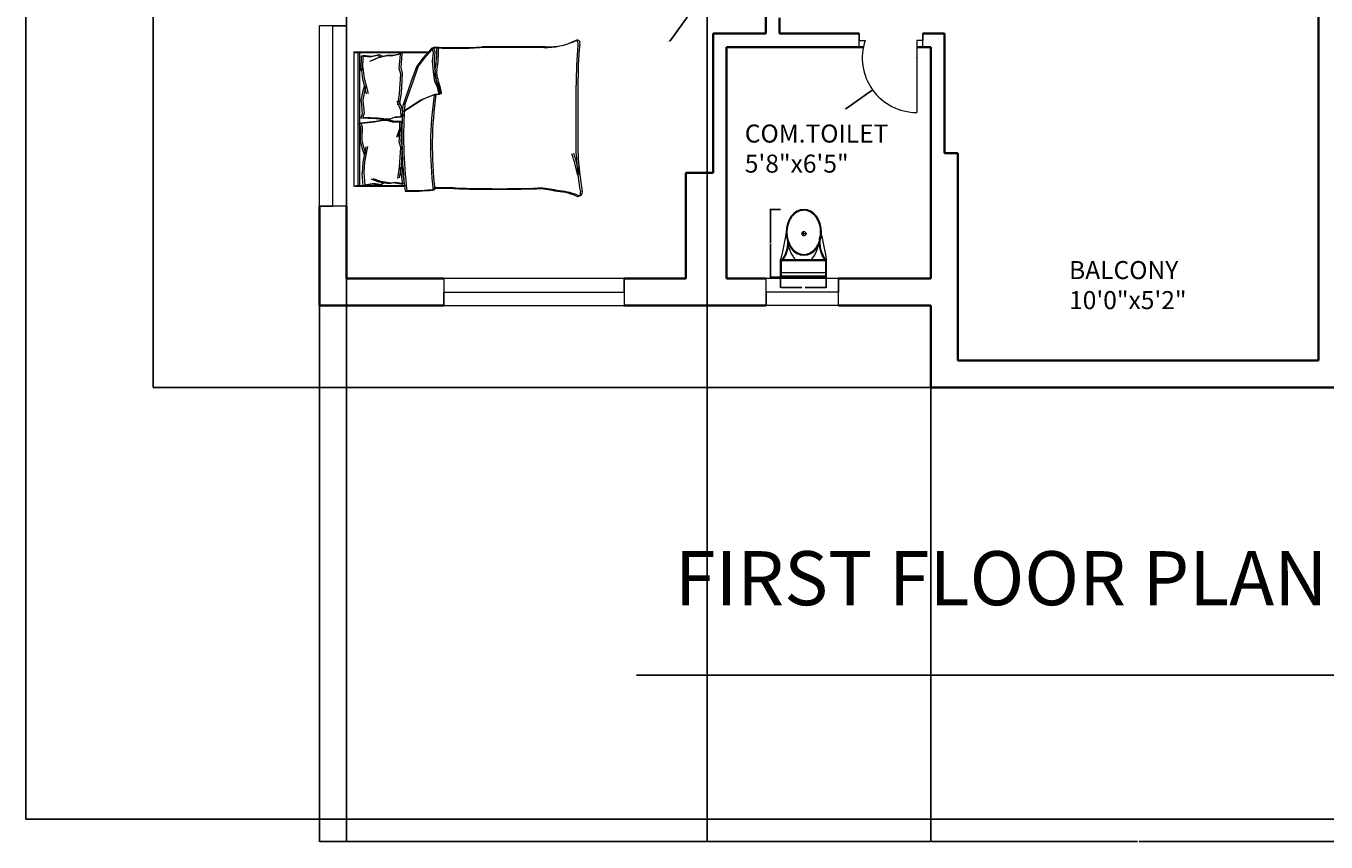
# Model space of a CAD drawing. Units: inches. Extents: x 1902 to 2626, y 1199 to 2408.
# Tile 1 of 9: x 1902 to 2334, y 1199 to 1470. Entities that reach past the tile are written whole.
import ezdxf

# ---------------------------------------------------------------- set-up
doc = ezdxf.new("R2010")
doc.units = ezdxf.units.IN
for name, color, linetype, lineweight in [('A-ANNO-DIMS', 2, 'Continuous', 18), ('A-ANNO-TTLB', 7, 'Continuous', 25), ('A-AREA-IDEN', 7, 'Continuous', 18), ('A-DOOR', 31, 'Continuous', 18), ('A-FLOR-FIXT', 9, 'Continuous', 18), ('A-FURN', 8, 'Continuous', 13), ('A-GLAZ', 181, 'Continuous', 18), ('A-WALL', 7, 'Continuous', 35)]:
    doc.layers.add(name, color=color, linetype=linetype, lineweight=lineweight)
doc.styles.get("Standard").update_dxf_attribs({"font": 'arial.ttf'})
doc.dimstyles.get("Standard").update_dxf_attribs({"dimtxt": 0.18, "dimasz": 0.18, "dimexe": 0.18, "dimexo": 0.0625, "dimgap": 0.09, "dimtad": 0, "dimtih": 1, "dimtoh": 1, "dimdec": 4, "dimzin": 0, "dimdsep": 46, "dimtxsty": 'Standard', "dimcen": 0.09, "dimadec": 0, "dimazin": 0, "dimtfac": 1, "dimtdec": 4, "dimtofl": 0, "dimtmove": 0, "dimatfit": 3, "dimfxl": 1, "dimtolj": 1, "dimtzin": 0, "dimarcsym": 0})

# ---------------------------------------------------------------- blocks, each defined once
blk = doc.blocks.new('A$C31115884')
for p, q in [((283, 498), (223, 498)), ((258, 466), (258, 523)), ((0, 200), (0, 0)), ((520, 200), (0, 200)), ((10, 190), (10, 10)), ((510, 190), (10, 190)), ((510, 10), (510, 190)), ((520, 0), (520, 200)), ((510, 54), (0, 54)), ((10, 10), (510, 10)), ((0, 0), (520, 0))]:
    blk.add_line(p, q)
blk.add_circle((256, 496), 23.6)
for centre, radius, start, end in [((2778, -205), 2807, 165.4549, 171.7133), ((-295, 403), 365, 324.2091, 9.3499), ((-295, 403), 375, 324.2091, 9.3499), ((806, 403), 365, 170.6501, 215.7909), ((3237, 905), 2807, 188.2867, 194.5451), ((384, 406), 293, 190.2774, 224.1564), ((139, 406), 293, 315.8436, 2.6563), ((806, 403), 375, 179.2036, 215.7909)]:
    blk.add_arc(centre, radius, start, end)
blk.add_ellipse((256, 510), major_axis=(0, -261), ratio=0.772727)
blk.add_open_spline([(256, 259), (263, 259), (270, 260), (288, 262), (299, 265), (320, 273), (330, 278), (350, 291), (360, 299), (378, 316), (386, 326), (402, 347), (409, 358), (421, 383), (427, 395), (436, 422), (440, 436), (445, 465), (447, 480), (448, 509), (448, 524), (445, 553), (443, 568), (436, 596), (432, 610), (422, 636), (416, 649), (402, 672), (395, 683), (379, 703), (370, 712), (351, 728), (341, 735), (321, 746), (310, 751), (289, 757), (278, 759), (256, 761), (245, 761), (223, 757), (212, 754), (191, 746), (181, 741), (161, 728), (151, 720), (133, 703), (125, 693), (110, 672), (103, 660), (90, 636), (85, 623), (76, 596), (72, 582), (67, 553), (66, 538), (64, 509), (65, 494), (68, 465), (70, 450), (77, 422), (81, 408), (91, 382), (97, 370), (111, 346), (118, 335), (135, 316), (144, 307), (162, 291), (172, 284), (193, 273), (203, 269), (225, 262), (236, 260), (250, 259), (253, 259), (256, 259)], degree=3, knots=[0, 0, 0, 0, 0.110105, 0.110105, 0.285049, 0.285049, 0.459994, 0.459994, 0.634938, 0.634938, 0.809882, 0.809882, 0.984827, 0.984827, 1.159771, 1.159771, 1.334715, 1.334715, 1.50966, 1.50966, 1.684604, 1.684604, 1.859549, 1.859549, 2.034493, 2.034493, 2.209437, 2.209437, 2.384382, 2.384382, 2.559326, 2.559326, 2.73427, 2.73427, 2.909215, 2.909215, 3.084159, 3.084159, 3.259103, 3.259103, 3.434048, 3.434048, 3.608992, 3.608992, 3.783936, 3.783936, 3.958881, 3.958881, 4.133825, 4.133825, 4.30877, 4.30877, 4.483714, 4.483714, 4.658658, 4.658658, 4.833603, 4.833603, 5.008547, 5.008547, 5.183491, 5.183491, 5.358436, 5.358436, 5.53338, 5.53338, 5.708324, 5.708324, 5.883269, 5.883269, 6.058213, 6.058213, 6.233158, 6.233158, 6.283185, 6.283185, 6.283185, 6.283185])
blk = doc.blocks.new('BED-DOUBLE')
for p, q in [((-0.01, 48.09), (0.59, 48.09)), ((-0.01, 48.09), (-0.01, 3.46)), ((-0.01, 47.87), (24.84, 47.87)), ((-0.01, 47.87), (24.84, 47.87)), ((0.59, 48.09), (25.44, 48.09)), ((0.59, 48.09), (25.44, 48.09)), ((1.43, 3.25), (1.43, 47.87)), ((1.43, 3.25), (1.43, 47.87)), ((2.02, 3.46), (2.02, 48.09)), ((2.02, 3.46), (2.02, 48.09)), ((25.9, 49.37), (22.87, 45.91)), ((25.9, 49.37), (22.87, 45.91)), ((26.5, 49.58), (23.46, 46.12)), ((26.5, 49.58), (23.46, 46.12)), ((27.53, 49.44), (25.9, 49.37, 3.61)), ((27.53, 49.44), (25.9, 49.37, 3.61)), ((26.48, 47.93), (25.9, 49.37)), ((26.48, 47.93), (25.9, 49.37)), ((26.19, 45.04), (26.48, 47.93)), ((26.19, 45.04), (26.48, 47.93)), ((28.13, 49.66), (26.5, 49.58, 3.61)), ((28.13, 49.66), (26.5, 49.58, 3.61)), ((27.08, 48.15), (26.5, 49.58)), ((27.08, 48.15), (26.5, 49.58)), ((26.79, 45.26), (27.08, 48.15)), ((26.79, 45.25), (27.08, 48.15)), ((2.38, 46.8), (2.29, 41.75)), ((2.38, 46.8), (2.29, 41.75)), ((2.38, 46.8), (5.38, 46.44)), ((2.38, 46.8), (5.38, 46.44)), ((2.98, 47.01), (2.89, 41.97)), ((2.98, 47.01), (2.89, 41.96)), ((2.98, 47.01), (5.98, 46.66)), ((2.98, 47.01), (5.98, 46.66)), ((7.7, 46.05), (5.2, 44.94)), ((7.7, 46.05), (5.2, 44.94)), ((5.38, 46.44), (7.78, 47)), ((5.38, 46.44), (7.78, 47)), ((8.3, 46.26), (5.8, 45.16)), ((8.3, 46.26), (5.8, 45.16)), ((5.98, 46.66), (8.38, 47.21)), ((5.98, 46.66), (8.38, 47.21)), ((11.04, 46.8), (7.7, 46.05)), ((11.04, 46.8), (7.7, 46.05)), ((7.78, 47), (8.76, 46.52)), ((7.78, 47), (8.76, 46.52)), ((11.64, 47.01), (8.3, 46.26)), ((11.64, 47.01), (8.3, 46.26)), ((8.38, 47.21), (9.35, 46.73)), ((8.38, 47.21), (9.35, 46.73)), ((12.54, 46.62), (11.04, 46.8)), ((12.54, 46.62), (11.04, 46.8)), ((13.14, 46.83), (11.64, 47.01)), ((13.14, 46.83), (11.64, 47.01)), ((15.47, 47.34), (12.54, 46.62)), ((15.47, 47.34), (12.54, 46.62)), ((16.07, 47.56), (13.14, 46.83)), ((16.07, 47.56), (13.14, 46.83)), ((15.09, 42.55), (15.47, 47.34)), ((15.09, 42.55), (15.47, 47.34)), ((15.69, 42.77), (16.07, 47.56)), ((15.69, 42.77), (16.07, 47.56)), ((21.44, 43.38), (19.56, 38.17)), ((21.44, 43.38), (19.56, 38.17)), ((22.87, 45.91), (20.84, 43.16)), ((22.87, 45.91), (20.84, 43.16)), ((23.46, 46.12), (21.44, 43.38)), ((23.46, 46.12), (21.44, 43.38)), ((26.48, 41.43), (26.19, 45.04)), ((26.48, 41.43), (26.19, 45.04)), ((27.08, 41.64), (26.79, 45.26)), ((27.08, 41.64), (26.79, 45.25)), ((2.29, 41.75), (2.37, 42.69)), ((2.29, 41.75), (2.37, 42.69)), ((2.37, 42.69), (2.86, 39.14)), ((2.37, 42.69), (2.86, 39.14)), ((2.86, 39.14), (4.12, 34.08)), ((2.86, 39.14), (4.12, 34.08)), ((2.89, 41.97), (2.97, 42.9)), ((2.89, 41.96), (2.97, 42.9)), ((2.97, 42.9), (3.46, 39.36)), ((2.97, 42.9), (3.46, 39.35)), ((3.46, 39.36), (4.72, 34.29)), ((3.46, 39.35), (4.72, 34.29)), ((15.61, 40.72), (15.09, 42.55)), ((15.61, 40.72), (15.09, 42.55)), ((15.21, 34.18), (15.61, 40.72)), ((15.21, 34.18), (15.61, 40.72)), ((16.21, 40.93), (15.69, 42.77)), ((16.21, 40.93), (15.69, 42.77)), ((15.81, 34.39), (16.21, 40.93)), ((15.81, 34.39), (16.21, 40.93)), ((20.84, 43.16), (18.97, 37.96)), ((20.84, 43.16), (18.97, 37.96)), ((26.91, 38.25), (26.48, 41.43)), ((26.91, 38.24), (26.48, 41.43)), ((27.51, 38.46), (27.08, 41.64)), ((27.51, 38.46), (27.08, 41.64)), ((2.87, 34.68), (2.36, 31.94)), ((2.87, 34.68), (2.36, 31.94)), ((3.42, 36.61), (2.87, 34.68)), ((3.42, 36.61), (2.87, 34.68)), ((3.47, 34.89), (2.96, 32.16)), ((3.47, 34.89), (2.96, 32.16)), ((4.02, 36.82), (3.47, 34.89)), ((4.02, 36.82), (3.47, 34.89)), ((18.97, 37.96), (16.23, 30.17)), ((18.97, 37.96), (16.23, 30.17)), ((19.56, 38.17), (16.82, 30.38)), ((19.56, 38.17), (16.82, 30.38)), ((27.78, 36.37), (26.91, 38.25)), ((27.78, 36.36), (26.91, 38.24)), ((28.38, 36.58), (27.51, 38.46)), ((28.38, 36.58), (27.51, 38.46)), ((28.36, 34.05), (27.78, 36.37)), ((28.36, 34.05), (27.78, 36.36)), ((28.96, 34.26), (28.38, 36.58)), ((28.96, 34.26), (28.38, 36.58)), ((73.99, 14.07), (73.99, 37.05)), ((73.99, 14.07), (73.99, 37.05)), ((74.59, 14.28), (74.59, 37.27)), ((74.59, 14.28), (74.59, 37.27)), ((2.36, 31.94), (2.38, 31.64)), ((2.36, 31.94), (2.38, 31.64)), ((2.38, 31.64), (2.78, 27.51)), ((2.38, 31.64), (2.78, 27.51)), ((2.96, 32.16), (2.98, 31.86)), ((2.96, 32.16), (2.98, 31.86)), ((2.98, 31.86), (3.37, 27.72)), ((2.98, 31.86), (3.37, 27.72)), ((15.63, 28.72), (14.43, 31.58)), ((15.63, 28.72), (14.43, 31.58)), ((14.59, 30.41), (15.21, 34.18)), ((14.59, 30.41), (15.21, 34.18)), ((16.22, 28.93), (15.02, 31.8)), ((16.22, 28.93), (15.02, 31.8)), ((15.18, 30.62), (15.81, 34.39)), ((15.18, 30.62), (15.81, 34.39)), ((16.23, 28.26), (22.29, 32.17)), ((16.23, 28.26), (22.29, 32.17)), ((16.82, 28.47), (22.89, 32.38)), ((16.82, 28.47), (22.89, 32.38)), ((22.29, 32.17), (26.48, 33.76)), ((22.29, 32.17), (26.48, 33.76)), ((22.89, 32.38), (27.08, 33.98)), ((22.89, 32.38), (27.08, 33.98)), ((26.48, 33.76), (28.36, 34.05)), ((26.48, 33.76), (28.36, 34.05)), ((27.08, 33.98), (28.96, 34.26)), ((27.08, 33.98), (28.96, 34.26)), ((2.78, 27.51), (2.32, 26.13)), ((2.78, 27.51), (2.32, 26.13)), ((2.32, 26.13), (7.34, 25.9)), ((2.32, 26.13), (7.34, 25.9)), ((3.37, 27.72), (2.92, 26.34)), ((3.37, 27.72), (2.92, 26.34)), ((2.92, 26.34), (7.94, 26.11)), ((2.92, 26.34), (7.94, 26.11)), ((7.94, 26.11), (10.94, 25.76)), ((7.94, 26.11), (10.94, 25.76)), ((11.55, 25.62), (13.27, 26.27)), ((11.55, 25.62), (13.27, 26.27)), ((12.15, 25.84), (13.87, 26.48)), ((12.15, 25.84), (13.87, 26.48)), ((13.27, 26.27), (15.77, 26.43)), ((13.27, 26.27), (15.77, 26.43)), ((13.87, 26.48), (16.37, 26.64)), ((13.87, 26.48), (16.37, 26.64)), ((15.77, 26.43), (15.63, 28.72)), ((15.77, 26.43), (15.63, 28.72)), ((16.37, 26.64), (16.22, 28.93)), ((16.37, 26.64), (16.22, 28.93)), ((1.74, 24.27), (6.74, 24.81)), ((1.74, 24.27), (6.74, 24.81)), ((2.28, 22.92), (1.74, 24.27)), ((2.28, 22.92), (1.74, 24.27)), ((2.15, 18.76), (2.28, 22.92)), ((2.15, 18.76), (2.28, 22.92)), ((2.34, 24.48), (7.33, 25.02)), ((2.34, 24.48), (7.33, 25.02)), ((2.88, 23.13), (2.34, 24.48)), ((2.88, 23.13), (2.34, 24.48)), ((2.74, 18.98), (2.88, 23.13)), ((2.74, 18.98), (2.88, 23.13)), ((6.74, 24.81), (9.71, 25.35)), ((6.74, 24.81), (9.71, 25.35)), ((7.33, 25.02), (10.3, 25.56)), ((7.33, 25.02), (10.3, 25.56)), ((7.34, 25.9), (10.34, 25.55)), ((7.34, 25.9), (10.34, 25.55)), ((9.71, 25.35), (10.92, 25.35)), ((9.71, 25.35), (10.92, 25.35)), ((10.3, 25.56), (11.52, 25.56)), ((10.3, 25.56), (11.52, 25.56)), ((10.34, 25.55), (11.55, 25.62)), ((10.34, 25.55), (11.55, 25.62)), ((10.92, 25.35), (12.68, 24.81)), ((10.92, 25.35), (12.68, 24.81)), ((10.94, 25.76), (12.15, 25.84)), ((10.94, 25.76), (12.15, 25.84)), ((11.52, 25.56), (13.27, 25.02)), ((11.52, 25.56), (13.27, 25.02)), ((12.68, 24.81), (15.18, 24.81)), ((12.68, 24.81), (15.18, 24.81)), ((13.27, 25.02), (15.78, 25.02)), ((13.27, 25.02), (15.78, 25.02)), ((15.18, 22.51), (14.16, 19.57)), ((15.18, 22.51), (14.16, 19.57)), ((15.78, 22.72), (14.76, 19.79)), ((15.78, 22.72), (14.76, 19.79)), ((15.09, 18.1), (15.47, 22.9)), ((15.09, 18.1), (15.47, 22.9)), ((15.18, 24.81), (15.18, 22.51)), ((15.18, 24.81), (15.18, 22.51)), ((15.69, 18.32), (16.07, 23.11)), ((15.69, 18.32), (16.07, 23.11)), ((15.78, 25.02), (15.78, 22.72)), ((15.78, 25.02), (15.78, 22.72)), ((2.15, 18.46), (2.15, 18.76)), ((2.15, 18.46), (2.15, 18.76)), ((2.82, 15.76), (2.15, 18.46)), ((2.82, 15.76), (2.15, 18.46)), ((2.74, 18.68), (2.74, 18.98)), ((2.74, 18.68), (2.74, 18.98)), ((3.42, 15.98), (2.74, 18.68)), ((3.42, 15.98), (2.74, 18.68)), ((15.61, 16.27), (15.09, 18.1)), ((15.61, 16.27), (15.09, 18.1)), ((16.21, 16.49), (15.69, 18.32)), ((16.21, 16.49), (15.69, 18.32)), ((3.5, 13.88), (2.82, 15.76)), ((3.5, 13.87), (2.82, 15.76)), ((3.09, 11.31), (4.04, 16.44)), ((3.09, 11.31), (4.04, 16.44)), ((4.09, 14.09), (3.42, 15.98)), ((4.09, 14.09), (3.42, 15.98)), ((3.69, 11.52), (4.63, 16.65)), ((3.69, 11.52), (4.63, 16.65)), ((15.21, 9.73), (15.61, 16.27)), ((15.21, 9.73), (15.61, 16.27)), ((15.81, 9.94), (16.21, 16.49)), ((15.81, 9.94), (16.21, 16.49)), ((2.82, 7.74), (3.09, 11.31)), ((2.82, 7.74), (3.09, 11.31)), ((3.42, 7.95), (3.69, 11.52)), ((3.42, 7.95), (3.69, 11.52)), ((14.59, 5.96), (15.21, 9.73)), ((14.59, 5.96), (15.21, 9.73)), ((15.18, 6.18), (15.81, 9.94)), ((15.18, 6.18), (15.81, 9.94)), ((15.21, 9.73), (15.51, 8.67)), ((15.21, 9.73), (15.51, 8.67)), ((15.51, 8.67), (16.19, 3.91)), ((15.51, 8.67), (16.19, 3.91)), ((15.81, 9.94), (16.11, 8.88)), ((15.81, 9.94), (16.11, 8.88)), ((16.11, 8.88), (16.78, 4.12)), ((16.11, 8.88), (16.78, 4.12)), ((2.8, 7.64), (2.82, 7.74)), ((2.8, 7.64), (2.82, 7.74)), ((3.11, 3.64), (2.8, 7.64)), ((3.11, 3.64), (2.8, 7.64)), ((3.4, 7.86), (3.42, 7.95)), ((3.4, 7.86), (3.42, 7.95)), ((3.71, 3.86), (3.4, 7.86)), ((3.71, 3.86), (3.4, 7.86)), ((3.69, 3.85), (6.66, 4.39)), ((3.69, 3.85), (6.66, 4.39)), ((8.36, 4.72), (5.79, 5.67)), ((8.36, 4.72), (5.79, 5.67)), ((8.95, 4.93), (6.39, 5.88)), ((8.95, 4.93), (6.39, 5.88)), ((6.66, 4.39), (9.09, 3.99)), ((6.66, 4.39), (9.09, 3.99)), ((11.73, 4.18), (8.36, 4.72)), ((11.73, 4.18), (8.36, 4.72)), ((12.33, 4.39), (8.95, 4.93)), ((12.33, 4.39), (8.95, 4.93)), ((9.09, 3.99), (10.03, 4.53)), ((9.09, 3.99), (10.03, 4.53)), ((13.22, 4.45), (11.73, 4.18)), ((13.22, 4.45), (11.73, 4.18)), ((13.81, 4.66), (12.33, 4.39)), ((13.81, 4.66), (12.33, 4.39)), ((16.19, 3.91), (13.22, 4.45)), ((16.19, 3.91), (13.22, 4.45)), ((16.78, 4.12), (13.81, 4.66)), ((16.78, 4.12), (13.81, 4.66)), ((16.91, 3.25), (-0.01, 3.25)), ((16.91, 3.25), (-0.01, 3.25)), ((17.5, 3.46), (0.59, 3.46)), ((17.5, 3.46), (0.59, 3.46)), ((3.09, 3.64), (6.06, 4.18)), ((3.09, 3.64), (6.06, 4.18)), ((6.06, 4.18), (8.49, 3.78)), ((6.06, 4.18), (8.49, 3.78)), ((8.49, 3.78), (9.44, 4.32)), ((8.49, 3.78), (9.44, 4.32))]:
    blk.add_line(p, q)
for centre, radius, start, end in [((64.71, 71.33), 21.54, 267.4714, 296.4681), ((64.71, 71.33), 21.54, 267.4714, 296.4681), ((74.24, 51.02), 1.03, 332.6588, 86.02), ((74.24, 51.02), 1.03, 332.6588, 86.02), ((-6.22, 47.93), 33.79, 349.8763, 2.5657), ((-6.22, 47.93), 33.79, 349.8763, 2.5657), ((33.9, 170.19), 120.92, 266.9791, 273.8365), ((33.9, 170.19), 120.92, 266.9791, 273.8365), ((-5.62, 48.14), 33.79, 349.8763, 2.5657), ((-5.62, 48.14), 33.79, 349.8763, 2.5657), ((34.5, 170.41), 120.92, 266.9791, 273.8365), ((34.5, 170.41), 120.92, 266.9791, 273.8365), ((63.32, -4210.02), 4259.62, 90.00217, 90.28689), ((63.32, -4210.02), 4259.62, 90.00217, 90.28689), ((63.92, -4209.8), 4259.62, 90.00217, 90.28689), ((63.92, -4209.8), 4259.62, 90.00217, 90.28689), ((64.11, 71.12), 21.54, 267.4714, 296.4681), ((64.11, 71.12), 21.54, 267.4714, 296.4681), ((73.64, 50.81), 1.03, 332.6588, 86.02), ((73.64, 50.81), 1.03, 332.6588, 86.02), ((198.21, 38.43), 124.23, 174.4998, 180.6351), ((198.21, 38.43), 124.23, 174.4998, 180.6351), ((198.8, 38.64), 124.23, 174.4998, 180.6351), ((198.8, 38.64), 124.23, 174.4998, 180.6351), ((32.74, 40.85), 5.81, 168.6608, 203.7384), ((32.74, 40.85), 5.81, 168.6608, 203.7384), ((33.33, 41.06), 5.81, 168.6608, 203.7384), ((33.33, 41.06), 5.81, 168.6608, 203.7384), ((1.38, 29.09), 27.69, 10.6617, 19.8806), ((1.38, 29.09), 27.69, 10.6617, 19.8806), ((1.98, 29.31), 27.69, 10.6617, 19.8806), ((1.98, 29.31), 27.69, 10.6617, 19.8806), ((169.99, 19.95), 154.04, 176.0865, 186.7821), ((169.99, 19.95), 154.04, 176.0865, 186.7821), ((170.58, 20.16), 154.04, 176.0865, 186.7821), ((170.58, 20.16), 154.04, 176.0865, 186.7821), ((145.95, 16.58), 120.47, 171.7845, 186.9006), ((145.95, 16.58), 120.47, 171.7845, 186.9006), ((146.55, 16.8), 120.47, 171.7845, 186.9006), ((146.55, 16.8), 120.47, 171.7845, 186.9006), ((28.42, 34.21), 0.172, 250.2464, 1.1377), ((28.42, 34.21), 0.172, 250.2464, 1.1377), ((29.01, 34.43), 0.172, 250.2464, 1.1377), ((29.01, 34.43), 0.172, 250.2464, 1.1377), ((-22.15, -16.08), 99.41, 13.3832, 17.7053), ((-22.15, -16.08), 99.41, 13.3832, 17.7053), ((-21.55, -15.86), 99.41, 13.3832, 17.7053), ((-21.55, -15.86), 99.41, 13.3832, 17.7053), ((187.53, 20.01), 113.69, 182.9958, 189.4091), ((187.53, 20.01), 113.69, 182.9958, 189.4091), ((188.12, 20.22), 113.69, 182.9958, 189.4091), ((188.12, 20.22), 113.69, 182.9958, 189.4091), ((18.76, 79.52), 77.79, 268.7218, 275.604), ((18.76, 79.52), 77.79, 268.7218, 275.604), ((19.36, 79.74), 77.79, 268.7218, 275.604), ((19.36, 79.74), 77.79, 268.7218, 275.604), ((29.1, -156.22), 158.84, 88.4762, 91.0082), ((29.1, -156.22), 158.84, 88.4762, 91.0082), ((29.7, -156), 158.84, 88.4762, 91.0082), ((29.7, -156.01), 158.84, 88.4762, 91.0082), ((47.26, 452.71), 450.36, 268.2277, 271.7185), ((47.26, 452.71), 450.36, 268.2277, 271.7185), ((47.85, 452.92), 450.36, 268.2277, 271.7185), ((47.85, 452.92), 450.36, 268.2277, 271.7185), ((60.24, -25.11), 27.67, 76.0648, 88.9113), ((60.24, -25.11), 27.67, 76.0648, 88.9113), ((60.83, -24.9), 27.67, 76.0648, 88.9113), ((60.83, -24.9), 27.67, 76.0648, 88.9113), ((65.61, -20.22), 22, 67.9751, 86.652), ((65.61, -20.22), 22, 67.9751, 86.652), ((66.21, -20.01), 22, 67.9751, 86.652), ((66.21, -20.01), 22, 67.9751, 86.652), ((74.43, 1.02), 1.02, 236.1736, 23.4781), ((74.43, 1.02), 1.02, 236.1736, 23.4781), ((75.03, 1.23), 1.02, 236.1736, 23.4781), ((75.03, 1.23), 1.02, 236.1736, 23.4781)]:
    blk.add_arc(centre, radius, start, end)
blk = doc.blocks.new('WINDOW-60-A')
for p, q in [((0, 9), (0, 0)), ((60, 9), (0, 9)), ((60, 4.5), (60, 9)), ((60, 9), (60, 0)), ((0, 0), (0, 4.5)), ((0, 4.5), (60, 4.5)), ((0, 0), (60, 0))]:
    blk.add_line(p, q)
blk = doc.blocks.new('WINDOW-24')
for p, q in [((0, 24), (9, 24)), ((0, 24), (0, 0)), ((9, 24), (4.5, 24)), ((4.5, 24), (4.5, 0)), ((9, 24), (9, 0)), ((4.5, 0), (0, 0)), ((0, 0), (9, 0))]:
    blk.add_line(p, q)
blk = doc.blocks.new('*D22')
at = {"layer": 'A-ANNO-DIMS', "color": 0, "lineweight": -2, "transparency": 16777216}
for p, q in [((2152.78, 1409.19), (2149.28, 1409.19)), ((2149.46, 1409.01), (2149.46, 1398.1)), ((2149.46, 1386.83), (2149.46, 1397.74)), ((2152.78, 1386.65), (2149.28, 1386.65))]:
    blk.add_line(p, q, dxfattribs=at)
at = {"layer": 'A-ANNO-DIMS', "color": 0, "transparency": 16777216}
for points in [[(2149.43, 1409.01), (2149.49, 1409.01), (2149.46, 1409.19)], [(2149.43, 1386.83), (2149.49, 1386.83), (2149.46, 1386.65)]]:
    blk.add_solid(points, dxfattribs=at)
at = {"layer": 'Defpoints', "color": 0, "transparency": 16777216}
for p in [(2149.46, 1409.19), (2152.84, 1409.19), (2152.84, 1386.65)]:
    blk.add_point(p, dxfattribs=at)
at = {"layer": 'A-ANNO-DIMS', "color": 0, "transparency": 16777216, "insert": (2149.46, 1397.92), "char_height": 0.18, "attachment_point": 5}
blk.add_mtext('\\A1;WC 23 TYP.', dxfattribs=at)
blk = doc.blocks.new('*D23')
at = {"layer": 'A-ANNO-DIMS', "color": 0, "lineweight": -2, "transparency": 16777216}
for p, q in [((2152.84, 1386.59), (2152.84, 1383.09)), ((2168.05, 1386.59), (2168.05, 1383.09)), ((2153.02, 1383.27), (2159.92, 1383.27)), ((2167.87, 1383.27), (2160.96, 1383.27))]:
    blk.add_line(p, q, dxfattribs=at)
at = {"layer": 'A-ANNO-DIMS', "color": 0, "transparency": 16777216}
for points in [[(2153.02, 1383.3), (2153.02, 1383.24), (2152.84, 1383.27)], [(2167.87, 1383.3), (2167.87, 1383.24), (2168.05, 1383.27)]]:
    blk.add_solid(points, dxfattribs=at)
at = {"layer": 'Defpoints', "color": 0, "transparency": 16777216}
for p in [(2152.84, 1386.65), (2168.05, 1386.65), (2152.84, 1383.27)]:
    blk.add_point(p, dxfattribs=at)
at = {"layer": 'A-ANNO-DIMS', "color": 0, "transparency": 16777216, "insert": (2160.44, 1383.27), "char_height": 0.18, "attachment_point": 5}
blk.add_mtext('\\A1;15 TYP.', dxfattribs=at)
blk = doc.blocks.new('*D29')
at = {"layer": 'A-ANNO-DIMS', "color": 0, "lineweight": -2, "transparency": 16777216}
for p, q in [((2191.29, 2322.47), (1943.87, 2322.47)), ((1944.05, 2322.29), (1944.05, 1836.38)), ((1944.05, 1350.11), (1944.05, 1836.02)), ((2202.79, 1349.93), (1943.87, 1349.93))]:
    blk.add_line(p, q, dxfattribs=at)
at = {"layer": 'A-ANNO-DIMS', "color": 0, "transparency": 16777216}
for points in [[(1944.02, 2322.29), (1944.08, 2322.29), (1944.05, 2322.47)], [(1944.02, 1350.11), (1944.08, 1350.11), (1944.05, 1349.93)]]:
    blk.add_solid(points, dxfattribs=at)
at = {"layer": 'Defpoints', "color": 0, "transparency": 16777216}
for p in [(1944.05, 2322.47), (2191.35, 2322.47), (2202.85, 1349.93)]:
    blk.add_point(p, dxfattribs=at)
at = {"layer": 'A-ANNO-DIMS', "color": 0, "transparency": 16777216, "insert": (1944.05, 1836.2), "char_height": 0.18, "attachment_point": 5}
blk.add_mtext('\\A1;972.5', dxfattribs=at)
blk = doc.blocks.new('*D30')
at = {"layer": 'A-ANNO-DIMS', "color": 0, "lineweight": -2, "transparency": 16777216}
for p, q in [((1999.35, 1377.14), (1999.35, 1198.67)), ((2202.85, 1349.87), (2202.85, 1198.67)), ((1999.53, 1198.85), (2100.7, 1198.85)), ((2202.67, 1198.85), (2101.5, 1198.85))]:
    blk.add_line(p, q, dxfattribs=at)
at = {"layer": 'A-ANNO-DIMS', "color": 0, "transparency": 16777216}
for points in [[(1999.53, 1198.88), (1999.53, 1198.82), (1999.35, 1198.85)], [(2202.67, 1198.88), (2202.67, 1198.82), (2202.85, 1198.85)]]:
    blk.add_solid(points, dxfattribs=at)
at = {"layer": 'Defpoints', "color": 0, "transparency": 16777216}
for p in [(1999.35, 1377.2), (2202.85, 1349.93), (2202.85, 1198.85)]:
    blk.add_point(p, dxfattribs=at)
at = {"layer": 'A-ANNO-DIMS', "color": 0, "transparency": 16777216, "insert": (2101.1, 1198.85), "char_height": 0.18, "attachment_point": 5}
blk.add_mtext('\\A1;203.5', dxfattribs=at)
blk = doc.blocks.new('*D31')
at = {"layer": 'A-ANNO-DIMS', "color": 0, "lineweight": -2, "transparency": 16777216}
for p, q in [((2202.85, 1349.87), (2202.85, 1198.67)), ((2340.85, 1349.87), (2340.85, 1198.67)), ((2203.03, 1198.85), (2271.57, 1198.85)), ((2340.67, 1198.85), (2272.13, 1198.85))]:
    blk.add_line(p, q, dxfattribs=at)
at = {"layer": 'A-ANNO-DIMS', "color": 0, "transparency": 16777216}
for points in [[(2203.03, 1198.88), (2203.03, 1198.82), (2202.85, 1198.85)], [(2340.67, 1198.88), (2340.67, 1198.82), (2340.85, 1198.85)]]:
    blk.add_solid(points, dxfattribs=at)
at = {"layer": 'Defpoints', "color": 0, "transparency": 16777216}
for p in [(2202.85, 1349.93), (2340.85, 1349.93), (2340.85, 1198.85)]:
    blk.add_point(p, dxfattribs=at)
at = {"layer": 'A-ANNO-DIMS', "color": 0, "transparency": 16777216, "insert": (2271.85, 1198.85), "char_height": 0.18, "attachment_point": 5}
blk.add_mtext('\\A1;138', dxfattribs=at)
blk = doc.blocks.new('*D38')
at = {"layer": 'A-ANNO-DIMS', "color": 0, "lineweight": -2, "transparency": 16777216}
for p, q in [((2008.35, 1874.05), (2008.35, 1198.67)), ((2128.35, 1874.05), (2128.35, 1198.67)), ((2008.53, 1198.85), (2068.07, 1198.85)), ((2128.17, 1198.85), (2068.63, 1198.85))]:
    blk.add_line(p, q, dxfattribs=at)
at = {"layer": 'A-ANNO-DIMS', "color": 0, "transparency": 16777216}
for points in [[(2008.53, 1198.88), (2008.53, 1198.82), (2008.35, 1198.85)], [(2128.17, 1198.88), (2128.17, 1198.82), (2128.35, 1198.85)]]:
    blk.add_solid(points, dxfattribs=at)
at = {"layer": 'Defpoints', "color": 0, "transparency": 16777216}
for p in [(2008.35, 1874.11), (2128.35, 1874.11), (2128.35, 1198.85)]:
    blk.add_point(p, dxfattribs=at)
at = {"layer": 'A-ANNO-DIMS', "color": 0, "transparency": 16777216, "insert": (2068.35, 1198.85), "char_height": 0.18, "attachment_point": 5}
blk.add_mtext('\\A1;120', dxfattribs=at)
blk = doc.blocks.new('*D51')
at = {"layer": 'A-ANNO-DIMS', "color": 0, "lineweight": -2, "transparency": 16777216}
for p, q in [((2141.3, 1500.7), (2141.48, 1500.7)), ((2141.39, 1500.61), (2141.39, 1500.79)), ((2116.07, 1465.29), (2125.46, 1478.42)), ((2115.89, 1465.29), (2116.07, 1465.29))]:
    blk.add_line(p, q, dxfattribs=at)
at = {"layer": 'A-ANNO-DIMS', "color": 0, "transparency": 16777216}
blk.add_solid([(2125.44, 1478.44), (2125.49, 1478.4), (2125.57, 1478.57)], dxfattribs=at)
at = {"layer": 'Defpoints', "color": 0, "transparency": 16777216}
for p in [(2141.39, 1500.7), (2125.57, 1478.57)]:
    blk.add_point(p, dxfattribs=at)
at = {"layer": 'A-ANNO-DIMS', "color": 0, "transparency": 16777216, "insert": (2115.34, 1465.29), "char_height": 0.18, "attachment_point": 5}
blk.add_mtext('\\A1;R27.204', dxfattribs=at)
blk = doc.blocks.new('*D59')
at = {"layer": 'A-ANNO-DIMS', "color": 0, "lineweight": -2, "transparency": 16777216}
for p, q in [((2198.11, 1459.63), (2198.29, 1459.63)), ((2198.2, 1459.54), (2198.2, 1459.72)), ((2174.57, 1442.68), (2183.28, 1448.93)), ((2174.39, 1442.68), (2174.57, 1442.68))]:
    blk.add_line(p, q, dxfattribs=at)
at = {"layer": 'A-ANNO-DIMS', "color": 0, "transparency": 16777216}
blk.add_solid([(2183.27, 1448.95), (2183.3, 1448.9), (2183.43, 1449.03)], dxfattribs=at)
at = {"layer": 'Defpoints', "color": 0, "transparency": 16777216}
for p in [(2198.2, 1459.63), (2183.43, 1449.03)]:
    blk.add_point(p, dxfattribs=at)
at = {"layer": 'A-ANNO-DIMS', "color": 0, "transparency": 16777216, "insert": (2173.84, 1442.68), "char_height": 0.18, "attachment_point": 5}
blk.add_mtext('\\A1;R18.174', dxfattribs=at)

msp = doc.modelspace()

# ---------------------------------------------------------------- linework, layer by layer
at = {"layer": 'A-ANNO-TTLB'}
msp.add_line((2104.9287, 1254.1475), (2368.8083, 1254.1475), dxfattribs=at)
msp.add_lwpolyline([(1901.6928, 2408.1473), (2626.1646, 2408.1473), (2626.1646, 1206.3103), (1901.6928, 1206.3103)], close=True, dxfattribs=at)
at = {"layer": 'A-DOOR'}
for p, q in [((2178.9818, 1463.2028), (2178.9818, 1467.7028)), ((2178.9818, 1467.7028), (2178.9818, 1465.4528)), ((2200.1971, 1463.2028), (2200.1971, 1467.7028)), ((2200.1971, 1467.7028), (2200.1971, 1465.4528)), ((2178.9818, 1465.4528), (2180.9818, 1465.4528)), ((2200.1971, 1465.4528), (2198.1971, 1465.4528)), ((2198.1971, 1465.4528), (2198.1971, 1441.4528))]:
    msp.add_line(p, q, dxfattribs=at)
msp.add_arc((2198.1971, 1459.627), 18.1742, 161.303826, 270, dxfattribs=at)
at = {"layer": 'A-WALL'}
for p, q in [((2331.8507, 1561.9733), (2331.8507, 1404.4733)), ((2147.9363, 1474.2928), (2147.9363, 1467.7028)), ((2152.4363, 1467.7028), (2152.4363, 1472.9548)), ((2130.3507, 1463.2028), (2130.3507, 1467.7028)), ((2130.3507, 1467.7028), (2147.9363, 1467.7028)), ((2152.4363, 1467.7028), (2178.9818, 1467.7028)), ((2200.1971, 1467.7028), (2207.3507, 1467.7028)), ((2207.3507, 1467.7028), (2207.3507, 1463.2028)), ((2130.3507, 1463.2028), (2130.3507, 1421.4173)), ((2134.8507, 1386.2028), (2134.8507, 1463.2028)), ((2134.8507, 1463.2028), (2180.378, 1463.2028)), ((2198.1971, 1463.2028), (2202.8507, 1463.2028)), ((2202.8507, 1463.2028), (2202.8507, 1386.2028)), ((2207.3507, 1463.2028), (2207.3507, 1427.8818)), ((2207.3507, 1427.8818), (2211.8507, 1427.8818)), ((2211.8507, 1386.2028), (2211.8507, 1427.8818)), ((2121.3507, 1386.2028), (2121.3507, 1421.4173)), ((2121.3507, 1421.4173), (2130.3507, 1421.4173)), ((1999.3507, 1410.2482), (1999.3507, 1377.2028)), ((2008.3507, 1410.2482), (2008.3507, 1386.2028)), ((2331.8507, 1404.4733), (2331.8507, 1358.9322)), ((2040.7143, 1386.2028), (2008.3507, 1386.2028)), ((2121.3507, 1386.2028), (2100.7143, 1386.2028)), ((2148.0684, 1386.2028), (2134.8507, 1386.2028)), ((2202.8507, 1386.2028), (2172.0684, 1386.2028)), ((2211.8507, 1358.9322), (2211.8507, 1386.2028)), ((2211.8507, 1386.2028), (2211.8507, 1386.2028)), ((2211.8507, 1377.2028), (2211.8507, 1386.2028)), ((2040.7143, 1377.2028), (1999.3507, 1377.2028)), ((2148.0684, 1377.2028), (2100.7143, 1377.2028)), ((2202.8507, 1377.2028), (2172.0684, 1377.2028)), ((2202.8507, 1377.2028), (2202.8507, 1358.9322)), ((2202.8507, 1358.9322), (2202.8507, 1349.9322)), ((2331.8507, 1358.9322), (2211.8507, 1358.9322)), ((2202.8507, 1349.9322), (2331.8507, 1349.9322)), ((2331.8507, 1349.9322), (2340.8507, 1349.9322))]:
    msp.add_line(p, q, dxfattribs=at)

# ---------------------------------------------------------------- block references
at = {"layer": 'A-FLOR-FIXT', "xscale": -0.0292470664339069, "yscale": 0.0292470664339069, "zscale": 0.0292470664339069}
msp.add_blockref('A$C31115884', (2168.0462, 1386.653), dxfattribs=at)
at = {"layer": 'A-FURN'}
msp.add_blockref('BED-DOUBLE', (2010.8265, 1413.546), dxfattribs=at)
at = {"layer": 'A-GLAZ', "extrusion": (0, 0, -1), "zscale": -1, "rotation": 90}
for name, p in [('WINDOW-60-A', (-1999.3474, 1410.2522)), ('WINDOW-24', (-2148.0664, 1377.2021))]:
    msp.add_blockref(name, p, dxfattribs=at)
at = {"layer": 'A-GLAZ'}
msp.add_blockref('WINDOW-60-A', (2040.7183, 1377.1994), dxfattribs=at)

# ---------------------------------------------------------------- texts
at = {"layer": 'A-ANNO-TTLB', "insert": (2117.6607, 1295.4667), "char_height": 18, "attachment_point": 1}
msp.add_mtext_dynamic_manual_height_columns('FIRST FLOOR PLAN', width=461.905947, gutter_width=12.5, heights=[0], dxfattribs=at)
at = {"layer": 'A-AREA-IDEN', "char_height": 6, "attachment_point": 1}
for s, width, insert in [('COM.TOILET\\P5\'8"x6\'5"', 100.484654, (2140.9206, 1437.4516)), ('BALCONY\\P10\'0"x5\'2"', 148.238549, (2248.846, 1392.0147))]:
    msp.add_mtext_dynamic_manual_height_columns(s, width=width, gutter_width=12.5, heights=[0], dxfattribs=dict(at, insert=insert))

# ---------------------------------------------------------------- dimensions: what is measured, and where the dimension line sits
at = {"layer": 'A-ANNO-DIMS'}
dim = msp.add_linear_dim(base=(1944.0507, 2322.4733), p1=(2202.8507, 1349.9322), p2=(2191.3507, 2322.4733), angle=90, dimstyle='Standard', override={"dimdec": 1, "dimlfac": 1, "dimrnd": 0, "dimzin": 0, "dimdsep": 46, "dimlunit": 2}, dxfattribs=at)
dim.commit()
dim.dimension.update_dxf_attribs({"geometry": '*D29', "text_midpoint": (1944.0507, 1836.2028)})
for base, p1, p2, override, picture, middle in [((2128.3507, 1198.8475), (2008.3507, 1874.11), (2128.3507, 1874.11), {"dimdec": 0, "dimlfac": 1, "dimrnd": 0, "dimzin": 0, "dimdsep": 46, "dimlunit": 2}, '*D38', (2068.3507, 1198.8475)), ((2202.8507, 1198.8475), (1999.3507, 1377.2028), (2202.8507, 1349.9322), {"dimdec": 1, "dimlfac": 1, "dimrnd": 0, "dimzin": 0, "dimdsep": 46, "dimlunit": 2}, '*D30', (2101.1007, 1198.8475)), ((2340.8507, 1198.8475), (2202.8507, 1349.9322), (2340.8507, 1349.9322), {"dimdec": 0, "dimlfac": 1, "dimrnd": 0, "dimzin": 0, "dimdsep": 46, "dimlunit": 2}, '*D31', (2271.8507, 1198.8475))]:
    dim = msp.add_linear_dim(base=base, p1=p1, p2=p2, dimstyle='Standard', override=override, dxfattribs=at)
    dim.commit()
    dim.dimension.update_dxf_attribs({"geometry": picture, "text_midpoint": middle})
for center, mpoint, picture, middle in [((2141.3902, 1500.6974), (2125.5668, 1478.5688), '*D51', (2115.3434, 1465.2916)), ((2198.1971, 1459.627), (2183.4291, 1449.0341), '*D59', (2173.8389, 1442.6783))]:
    dim = msp.add_radius_dim(center=center, mpoint=mpoint, dimstyle='Standard', override={"dimdec": 3, "dimlfac": 1, "dimrnd": 0, "dimzin": 0, "dimdsep": 46, "dimlunit": 2}, dxfattribs=at)
    dim.commit()
    dim.dimension.update_dxf_attribs({"geometry": picture, "text_midpoint": middle, "dimtype": 164})
for base, p1, p2, angle, text, picture, middle in [((2149.4572, 1409.1899), (2152.8377, 1386.653), (2152.8377, 1409.1899), 90, 'WC <> TYP.', '*D22', (2149.4572, 1397.9214)), ((2152.8377, 1383.2724), (2168.0462, 1386.653), (2152.8377, 1386.653), 180, '<> TYP.', '*D23', (2160.442, 1383.2724))]:
    dim = msp.add_linear_dim(base=base, p1=p1, p2=p2, angle=angle, text=text, dimstyle='Standard', override={"dimdec": 0, "dimlfac": 1, "dimrnd": 0, "dimzin": 0, "dimdsep": 46, "dimlunit": 2}, dxfattribs=at)
    dim.commit()
    dim.dimension.update_dxf_attribs({"geometry": picture, "text_midpoint": middle})

doc.saveas('drawing.dxf')
